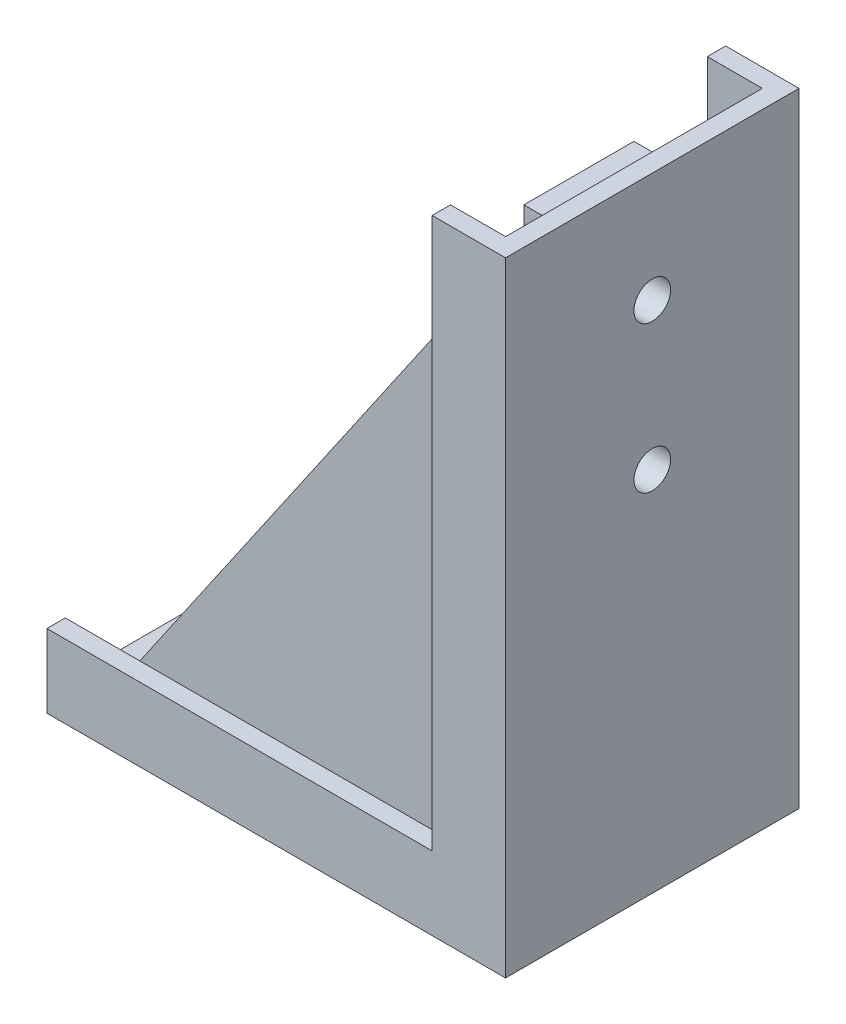
from build123d import *

# Parameters (mm, degrees)
BRACKET_L_BODY_DEPTH    = 20
LIP_FLANGE_DEPTH        = 1.25
END_PLATE_DEPTH         = 1.25
GUSSET_A_28_75X40_DEPTH = 1.25
GUSSET_B_27_5X40_DEPTH  = 1.25
TAB_AND_HOLES_SKETCH_W  = 7.5
TAB_AND_HOLES_SKETCH_H  = 22.5
TAB_AND_HOLES_SKETCH_R  = 1.25
MOUNTING_TAB_DEPTH      = 3.75
MOUNTING_START          = -3.75
SKETCH8_2_R             = 1.25
MOUNTING_HOLES_DEPTH    = 3.75


with BuildPart() as part:
    # L-Profile Sketch → Bracket L-Body (new body)
    with BuildSketch(Plane.XY):
        Polygon((0, 42.5), (0, 0), (-31.25, 0), (-31.25, 1.25), (-1.25, 1.25), (-1.25, 42.5), align=None)
    extrude(amount=BRACKET_L_BODY_DEPTH)

    # Lip Flange Sketch → Lip Flange (add)
    with BuildSketch(Plane.XY.offset(20)):
        Polygon((-1.25, 42.5), (-5, 42.5), (-5, 5), (-31.25, 5), (-31.25, 1.25), (-1.25, 1.25), align=None)
    extrude(amount=-LIP_FLANGE_DEPTH)

    # End Plate Sketch → End Plate (add)
    with BuildSketch(Plane(origin=(0, 0, 0), x_dir=(-1, 0, 0), z_dir=(0, 0, -1))):
        Polygon((0, 42.5), (1.25, 42.5), (5, 42.5), (5, 5), (31.25, 5), (31.25, 1.25), (31.25, 0), (0, 0), align=None)
    extrude(amount=-END_PLATE_DEPTH)

    # Gusset A Sketch → Gusset A 28.75x40 (add)
    with BuildSketch(Plane.XY.offset(1.25)):
        Polygon((-28.75, 1.25), (-1.25, 41.25), (-1.25, 1.25), align=None)
    extrude(amount=GUSSET_A_28_75X40_DEPTH)

    # Gusset B Sketch → Gusset B 27.5x40 (add)
    with BuildSketch(Plane(origin=(0, 0, 18.75), x_dir=(-1, 0, 0), z_dir=(0, 0, -1))):
        Polygon((1.25, 41.25), (28.75, 1.25), (1.25, 1.25), align=None)
    extrude(amount=GUSSET_B_27_5X40_DEPTH)

    # Tab And Holes Sketch → Mounting Tab (add)
    with BuildSketch(Plane.ZY.offset(1.25)):
        with Locations((10, 28.75)):
            Rectangle(TAB_AND_HOLES_SKETCH_W, TAB_AND_HOLES_SKETCH_H)
        with Locations(Location((10, 35, 0), (0, 0, 270))):
            Circle(TAB_AND_HOLES_SKETCH_R, mode=Mode.SUBTRACT)
        with Locations(Location((10, 25, 0), (0, 0, 270))):
            Circle(TAB_AND_HOLES_SKETCH_R, mode=Mode.SUBTRACT)
    extrude(amount=MOUNTING_TAB_DEPTH)

    # Sketch8_2 → Mounting Holes (cut)
    with BuildSketch(Plane.ZY.offset(1.25).offset(MOUNTING_START)):
        with Locations(Location((10, 35, 0), (0, 0, 270))):
            Circle(SKETCH8_2_R)
        with Locations(Location((10, 25, 0), (0, 0, 270))):
            Circle(SKETCH8_2_R)
    extrude(amount=MOUNTING_HOLES_DEPTH, mode=Mode.SUBTRACT)


solid = part.part
